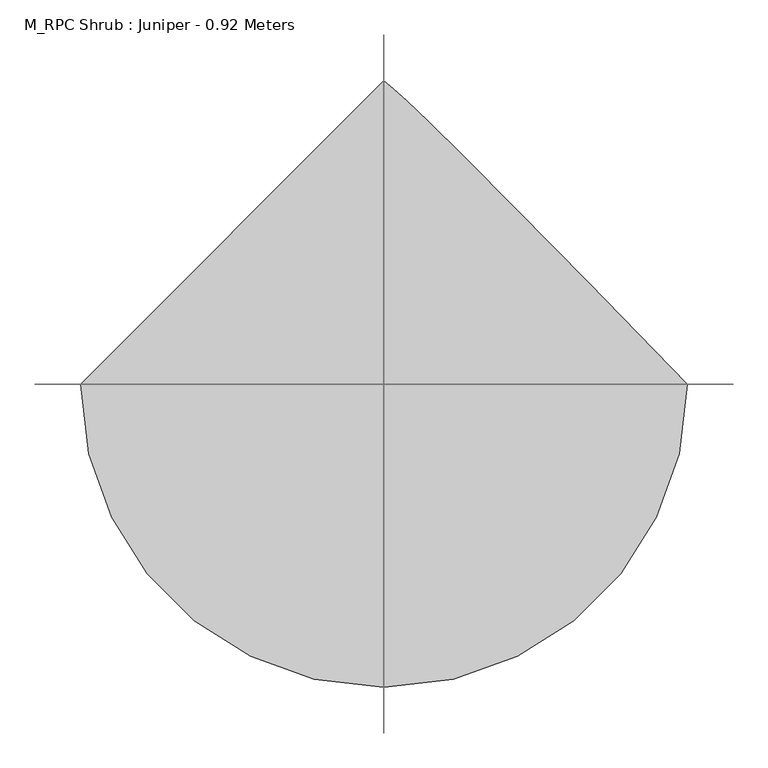
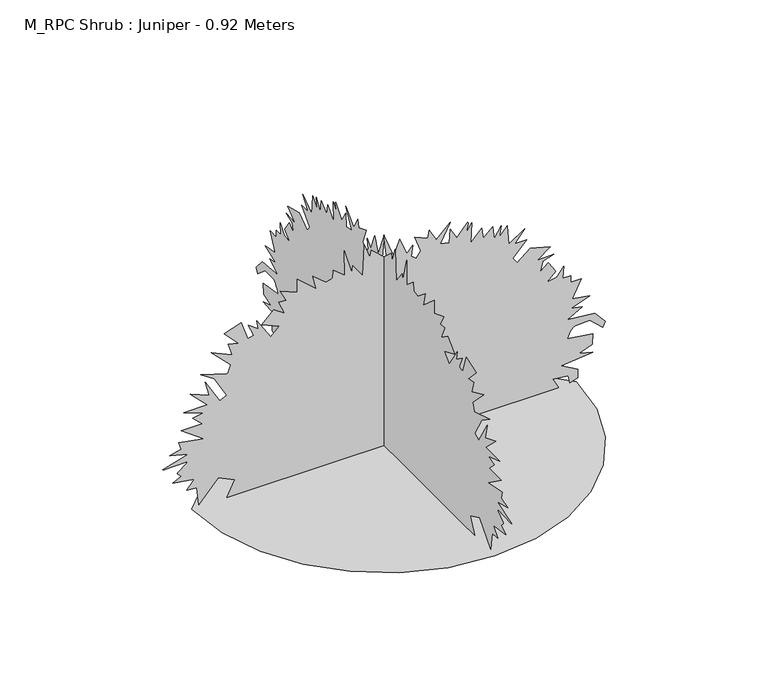
"""IFC4 building model written with IfcOpenShell, lengths in millimetres: geographic element geometry, M_RPC Shrub : Juniper - 0.92 Meters."""

from ifc_helpers import new_model, si_unit, origin, place, context, project, spatial, triangles, source, transform, mapped, element, save


def m_rpc_shrub_juniper_0_92_meters_8f64cf4e(model_context):
    return source(origin(), model_context, "Body", "Tessellation", [
        triangles([(-794.7784498, 0.0, 7.39e-05), (-773.7691944, -182.1108318, 7.39e-05), (-713.9282249, -349.3498243, 7.39e-05), (-620.0497982, -496.928171, 7.39e-05), (-496.928171, -620.0497982, 7.39e-05), (-349.3498243, -713.9282249, 7.39e-05), (-182.1108318, -773.7691944, 7.39e-05), (3.47e-05, -794.7784498, 7.39e-05), (182.1110862, -773.7691944, 7.39e-05), (349.3498243, -713.9282249, 7.39e-05), (496.928171, -620.0497982, 7.39e-05), (620.0497982, -496.928171, 7.39e-05), (713.9282249, -349.3498243, 7.39e-05), (773.7691944, -182.1108318, 7.39e-05), (794.7784498, 6.95e-05, 7.39e-05), (536.4933068, 264.9372079, 7.39e-05), (345.0130614, 460.0003741, 7.39e-05), (209.2048539, 596.8325744, 7.39e-05), (117.9336172, 687.0795731, 7.39e-05), (60.065061, 742.3894964, 7.39e-05), (24.4653762, 774.4080362, 7.39e-05), (-0.0001042, 794.7784498, 7.39e-05), (-3.6e-06, -649.9319859, 2.9e-06), (1e-06, -617.9951271, 67.2298217), (0.0, -685.063199, 99.2021479), (0.0, -764.9065086, 9.7766686), (0.0, -774.4898626, 86.4271646), (0.0, -816.0074593, 89.6208469), (0.0, -784.0706005, 127.946033), (0.0, -873.4947206, 140.7212706), (0.0, -838.3634348, 159.8838637), (0.0, -854.3330996, 175.8527654), (2e-07, -852.2145515, 179.4443521), (-1e-07, -815.0695078, 209.220696), (0.0, -812.8129595, 214.1779515), (2e-07, -908.8278111, 211.8641574), (0.0, -915.0148607, 214.1779515), (0.0, -809.6210758, 246.115537), (0.0, -886.2699583, 265.2771036), (0.0, -838.3634348, 278.0523412), (0.0, -847.9442453, 309.9916889), (0.0, -745.7449602, 290.8275607), (0.0, -838.3634348, 357.8981761), (0.0, -752.131271, 357.8981761), (0.0, -790.4569839, 396.2238891), (0.0, -745.7449602, 405.8046633), (0.0, -828.7826969, 434.5470222), (0.0, -729.7752228, 434.5470222), (0.0, -800.0377218, 504.8120647), (0.0, -723.388912, 472.8726989), (0.0, -739.3585768, 536.7488872), (0.0, -678.6743448, 434.5470222), (0.0, -649.9319859, 447.3222599), (0.0, -701.0328638, 536.7488872), (0.0, -758.5201979, 575.0745638), (0.0, -646.7374861, 539.9433143), (0.0, -633.9623211, 575.0745638), (0.0, -713.8081015, 654.9178734), (0.0, -627.5759377, 616.5921604), (0.0, -643.5456024, 667.693111), (0.0, -602.0254987, 658.1123005), (0.0, -659.5127237, 718.793989), (0.0, -589.250261, 744.3444643), (0.0, -563.6997857, 664.4986113), (0.0, -538.1493104, 670.8875381), (0.0, -560.5053223, 721.9859453), (0.0, -518.987762, 693.2435863), (6e-07, -525.3740727, 728.7095901), (0.0, -467.8868114, 638.9482086), (0.0, -432.7555618, 674.0794218), (0.0, -506.2125243, 706.0187513), (0.0, -455.1115737, 753.9252748), (0.0, -410.39955, 721.9859453), (0.0, -435.9500253, 779.4757502), (0.0, -404.0106594, 776.2813231), (0.0, -429.5611347, 824.1877739), (0.0, -359.2986357, 795.4428715), (0.0, -359.2986357, 852.9326763), (0.0, -279.4553261, 782.6676338), (0.0, -295.4224656, 843.3493223), (0.0, -241.1293769, 798.6372986), (0.0, -212.3857462, 805.0262255), (0.0, -209.1915553, 840.1574387), (0.0, -161.2850681, 801.8317257), (0.0, -164.4792591, 910.4199377), (0.0, -132.5414374, 801.8317257), (0.0, -129.3475008, 830.5740847), (0.0, -87.8283782, 773.0868233), (0.0, -81.4410228, 907.2255106), (0.0, -59.0844931, 843.3493223), (0.0, -52.6971332, 872.0942247), (0.0, 11.1781115, 814.6069633), (0.0, -1.5967073, 920.0007483), (0.0, 39.9224087, 814.6069633), (0.0, 65.4723617, 878.4806082), (0.0, 94.2162513, 805.0262255), (0.0, 119.7664632, 833.7685844), (0.0, 113.3788444, 789.056488), (0.0, 132.5416918, 773.0868233), (0.0, 151.7042848, 798.6372986), (0.0, 126.154082, 865.707914), (0.0, 180.448179, 843.3493223), (0.0, 186.8352891, 875.2887245), (0.0, 215.5796828, 824.1877739), (0.0, 273.0664355, 881.6750353), (0.0, 231.5483484, 801.8317257), (0.0, 269.8745519, 792.2509878), (0.0, 273.0664355, 849.7382492), (0.0, 301.8113561, 801.8317257), (0.0, 344.4942704, 854.0673454), (0.0, 346.8402755, 853.8730986), (0.0, 347.5124002, 849.9043728), (0.0, 340.1370509, 811.4125362), (0.0, 362.4930628, 846.5438221), (0.0, 359.2986357, 760.3115856), (0.0, 404.0132029, 808.2181091), (0.0, 410.39955, 763.5060854), (0.0, 448.7252629, 798.6372986), (0.0, 455.1115737, 744.3444643), (0.0, 483.8565125, 792.2509878), (0.0, 477.4676219, 744.3444643), (0.0, 509.4069514, 782.6676338), (0.0, 515.7932985, 699.6298971), (0.0, 582.8639139, 744.3444643), (0.0, 541.3437738, 693.2435863), (0.0, 589.250261, 693.2435863), (0.0, 531.7629633, 632.5618252), (0.0, 550.9245481, 607.0113862), (0.0, 605.2199258, 651.7234463), (0.0, 688.2576262, 629.3673981), (0.0, 633.9623211, 587.8498014), (0.0, 701.0328638, 591.0416851), (0.0, 656.3208401, 575.0745638), (0.0, 646.7374861, 533.5544237), (0.0, 678.6768883, 562.2993261), (0.0, 710.6136744, 514.392839), (0.0, 672.2879614, 479.2615894), (0.0, 713.8081015, 485.6479365), (0.0, 742.5504604, 523.9736495), (0.0, 739.3585768, 472.8726989), (0.0, 771.2953629, 472.8726989), (0.0, 771.2953629, 444.1303399), (0.0, 816.0074593, 444.1303399), (0.0, 777.6817463, 370.6734138), (0.0, 851.1386724, 357.8981761), (0.0, 774.4898626, 329.1532737), (0.0, 819.2018864, 319.5724631), (0.0, 758.5201979, 284.4412318), (0.0, 870.302837, 274.8604394), (0.0, 915.0148607, 223.7592526), (0.0, 905.4340502, 201.402732), (0.0, 851.1386724, 249.3092192), (0.0, 790.1144903, 247.912593), (0.0, 782.0312628, 244.0018215), (0.0, 775.4865314, 237.9960108), (0.0, 770.1683968, 230.3142667), (0.0, 765.7728075, 221.375441), (0.0, 761.993169, 211.5986395), (0.0, 758.5201979, 201.402732), (0.0, 863.9139101, 185.4340665), (0.0, 860.7220264, 140.7212706), (0.0, 806.4266487, 121.5586776), (0.0, 863.9139101, 105.5897668), (0.0, 732.9697226, 92.8147835), (0.0, 800.0403379, 54.489343), (0.0, 800.0403379, 16.164208), (0.0, 768.1009357, 6.582912), (0.0, 761.714625, 38.5206865), (0.0, 697.8384367, 44.9080465), (0.0, 723.388912, 0.1953706), (-649.9319859, 0.0001197, 0.0), (-617.9951271, 0.0001111, 67.2298217), (-685.063199, 0.0001102, 99.2021479), (-764.9065086, 0.0001155, 9.7766686), (-774.4898626, 0.0001109, 86.4271646), (-816.0074593, 0.0001107, 89.6208469), (-784.0706005, 0.0001084, 127.946033), (-873.4947206, 0.0001077, 140.7212706), (-838.3634348, 0.0001065, 159.8838637), (-854.3330996, 0.0001056, 175.8527654), (-852.2145515, 0.0001052, 179.4443521), (-815.0695078, 0.0001037, 209.220696), (-812.8129595, 0.0001033, 214.1779515), (-908.8278111, 0.0001032, 211.8641574), (-915.0148607, 0.0001033, 214.1779515), (-809.6210758, 0.0001014, 246.115537), (-886.2699583, 0.0001003, 265.2771036), (-838.3634348, 9.95e-05, 278.0523412), (-847.9442453, 9.76e-05, 309.9916889), (-745.7449602, 9.87e-05, 290.8275607), (-838.3634348, 9.47e-05, 357.8981761), (-752.131271, 9.47e-05, 357.8981761), (-790.4569839, 9.25e-05, 396.2238891), (-745.7449602, 9.19e-05, 405.8046633), (-828.7826969, 9.02e-05, 434.5470222), (-729.7752228, 9.02e-05, 434.5470222), (-800.0377218, 8.6e-05, 504.8095213), (-723.388912, 8.79e-05, 472.8726989), (-739.3585768, 8.41e-05, 536.7488872), (-678.6768883, 9.02e-05, 434.5470222), (-649.9319859, 8.94e-05, 447.3222599), (-701.0328638, 8.41e-05, 536.7488872), (-758.5201979, 8.18e-05, 575.0745638), (-646.7374861, 8.39e-05, 539.9433143), (-633.9623211, 8.18e-05, 575.0745638), (-713.8081015, 7.7e-05, 654.9178734), (-627.5759377, 7.93e-05, 616.5921604), (-643.5456024, 7.63e-05, 667.693111), (-602.0254987, 7.68e-05, 658.1123005), (-659.5127237, 7.32e-05, 718.793989), (-589.250261, 7.17e-05, 744.3444643), (-563.6997857, 7.65e-05, 664.4986113), (-538.1493104, 7.61e-05, 670.8875381), (-560.5053223, 7.3e-05, 721.9859453), (-518.987762, 7.48e-05, 693.2435863), (-525.3740727, 7.2e-05, 728.7095901), (-467.8868114, 7.8e-05, 638.9482086), (-432.7555618, 7.59e-05, 674.0794218), (-506.2125243, 7.4e-05, 706.0187513), (-455.1115737, 7.11e-05, 753.9252748), (-410.39955, 7.3e-05, 721.9859453), (-435.9500253, 6.96e-05, 779.4757502), (-404.0132029, 6.98e-05, 776.2813231), (-429.5611347, 6.69e-05, 824.1877739), (-359.2986357, 6.87e-05, 795.4428715), (-359.2986357, 6.52e-05, 852.9326763), (-279.4553261, 6.94e-05, 782.6676338), (-295.4224656, 6.58e-05, 843.3493223), (-241.1293769, 6.85e-05, 798.6372986), (-212.3857462, 6.81e-05, 805.0262255), (-209.1918097, 6.6e-05, 840.1574387), (-161.2850681, 6.83e-05, 801.8317257), (-164.4792591, 6.18e-05, 910.4199377), (-132.5416918, 6.83e-05, 801.8317257), (-129.3475008, 6.66e-05, 830.5740847), (-87.8286325, 7e-05, 773.0868233), (-81.4410228, 6.2e-05, 907.2255106), (-59.0847475, 6.58e-05, 843.3493223), (-52.6973875, 6.41e-05, 872.0942247), (11.1780093, 6.75e-05, 814.6069633), (-1.5967993, 6.12e-05, 920.0007483), (39.9221544, 6.75e-05, 814.6069633), (65.4723617, 6.37e-05, 878.4806082), (94.2162513, 6.81e-05, 805.0262255), (119.7664632, 6.64e-05, 833.7685844), (113.3788444, 6.9e-05, 789.056488), (132.5414374, 7e-05, 773.0868233), (151.7040305, 6.85e-05, 798.6372986), (126.154082, 6.45e-05, 865.7053705), (180.4479246, 6.58e-05, 843.3493223), (186.8352891, 6.39e-05, 875.2887245), (215.5794285, 6.69e-05, 824.1877739), (273.0664355, 6.35e-05, 881.6750353), (231.5483484, 6.83e-05, 801.8317257), (269.8745519, 6.89e-05, 792.2509878), (273.0664355, 6.54e-05, 849.7382492), (301.8113561, 6.83e-05, 801.8317257), (344.4942704, 6.52e-05, 854.0673454), (346.8402755, 6.52e-05, 853.8730986), (347.5098204, 6.54e-05, 849.9043728), (340.1370509, 6.77e-05, 811.4125362), (362.4930628, 6.56e-05, 846.5438221), (359.2986357, 7.08e-05, 760.3115856), (404.0106594, 6.79e-05, 808.2181091), (410.39955, 7.06e-05, 763.5060854), (448.7252629, 6.85e-05, 798.6372986), (455.1115737, 7.17e-05, 744.3444643), (483.8565125, 6.89e-05, 792.2509878), (477.4676219, 7.17e-05, 744.3444643), (509.4069514, 6.94e-05, 782.6676338), (515.7932985, 7.44e-05, 699.6298971), (582.8639139, 7.17e-05, 744.3444643), (541.3437738, 7.48e-05, 693.2435863), (589.250261, 7.48e-05, 693.2435863), (531.7629633, 7.84e-05, 632.5618252), (550.9245481, 7.99e-05, 607.0113862), (605.2199258, 7.72e-05, 651.7234463), (688.2576262, 7.86e-05, 629.3673981), (633.9623211, 8.1e-05, 587.8498014), (701.0328638, 8.08e-05, 591.0416851), (656.3208401, 8.18e-05, 575.0745638), (646.7374861, 8.43e-05, 533.5544237), (678.6768883, 8.26e-05, 562.2993261), (710.6136744, 8.54e-05, 514.392839), (672.2879614, 8.75e-05, 479.2615894), (713.8081015, 8.71e-05, 485.6479365), (742.5504604, 8.48e-05, 523.9736495), (739.3585768, 8.79e-05, 472.8726989), (771.2953629, 8.79e-05, 472.8726989), (771.2953629, 8.96e-05, 444.1303399), (816.0074593, 8.96e-05, 444.1303399), (777.6817463, 9.4e-05, 370.6734138), (851.1386724, 9.47e-05, 357.8981761), (774.4898626, 9.65e-05, 329.1532737), (819.2018864, 9.7e-05, 319.5724631), (758.5201979, 9.91e-05, 284.4412318), (870.302837, 9.97e-05, 274.8604394), (915.0148607, 0.0001027, 223.7592526), (905.4340502, 0.0001041, 201.402732), (851.1386724, 0.0001012, 249.3092192), (790.1144903, 0.0001013, 247.912593), (782.0312628, 0.0001015, 244.0018215), (775.4865314, 0.0001019, 237.9960108), (770.1683968, 0.0001023, 230.3142667), (765.7728075, 0.0001029, 221.375441), (761.993169, 0.0001035, 211.5986395), (758.5201979, 0.0001041, 201.402732), (863.9139101, 0.000105, 185.4338121), (860.7220264, 0.0001077, 140.7212706), (806.4266487, 0.0001088, 121.5586776), (863.9139101, 0.0001098, 105.5897668), (732.9697226, 0.0001105, 92.8145291), (800.0403379, 0.0001128, 54.489343), (800.0403379, 0.0001151, 16.164208), (768.1009357, 0.0001157, 6.582912), (761.714625, 0.0001138, 38.5206865), (697.8384367, 0.0001134, 44.9080465), (723.388912, 0.0001161, 0.1953678)], [[21, 22, 1], [20, 21, 1], [19, 20, 1], [18, 19, 1], [17, 18, 1], [17, 1, 2], [17, 2, 3], [17, 3, 4], [16, 17, 4], [16, 4, 5], [16, 5, 6], [16, 6, 7], [16, 7, 8], [16, 8, 9], [16, 9, 10], [16, 10, 11], [16, 11, 12], [15, 16, 12], [14, 15, 12], [13, 14, 12], [92, 93, 94], [84, 85, 86], [54, 55, 56], [50, 51, 52], [131, 132, 133], [123, 124, 125], [104, 105, 106], [46, 47, 48], [57, 58, 59], [88, 89, 90], [48, 49, 50], [67, 68, 69], [119, 120, 121], [162, 163, 164], [38, 39, 40], [113, 114, 115], [144, 145, 146], [65, 66, 67], [138, 139, 140], [96, 97, 98], [107, 108, 109], [79, 80, 81], [42, 43, 44], [29, 30, 31], [36, 37, 38], [75, 76, 77], [102, 103, 104], [146, 147, 148], [86, 87, 88], [94, 95, 96], [121, 122, 123], [125, 126, 127], [100, 101, 102], [77, 78, 79], [25, 26, 27], [115, 116, 117], [129, 130, 131], [117, 118, 119], [27, 28, 29], [82, 83, 84], [44, 45, 46], [48, 50, 52], [59, 60, 61], [169, 170, 23], [73, 74, 75], [90, 91, 92], [142, 143, 144], [40, 41, 42], [38, 40, 42], [169, 23, 24], [53, 54, 56], [61, 62, 63], [61, 63, 64], [70, 71, 72], [70, 72, 73], [150, 151, 152], [149, 150, 152], [148, 149, 152], [148, 152, 153], [128, 129, 131], [148, 153, 154], [35, 36, 38], [134, 135, 136], [134, 136, 137], [65, 67, 69], [166, 167, 168], [165, 166, 168], [164, 165, 168], [164, 168, 169], [88, 90, 92], [140, 141, 142], [100, 102, 104], [159, 160, 161], [159, 161, 162], [25, 27, 29], [123, 125, 127], [148, 154, 155], [100, 104, 106], [110, 111, 112], [109, 110, 112], [109, 112, 113], [109, 113, 115], [31, 32, 33], [131, 133, 134], [159, 162, 164], [128, 131, 134], [46, 48, 52], [73, 75, 77], [73, 77, 79], [29, 31, 33], [29, 33, 34], [44, 46, 52], [148, 155, 156], [164, 169, 24], [159, 164, 24], [158, 159, 24], [157, 158, 24], [156, 157, 24], [148, 156, 24], [146, 148, 24], [144, 146, 24], [142, 144, 24], [140, 142, 24], [138, 140, 24], [137, 138, 24], [134, 137, 24], [128, 134, 24], [127, 128, 24], [123, 127, 24], [121, 123, 24], [119, 121, 24], [117, 119, 24], [115, 117, 24], [109, 115, 24], [107, 109, 24], [106, 107, 24], [106, 24, 25], [106, 25, 29], [106, 29, 34], [106, 34, 35], [106, 35, 38], [106, 38, 42], [106, 42, 44], [106, 44, 52], [106, 52, 53], [106, 53, 56], [99, 100, 106], [99, 106, 56], [99, 56, 57], [98, 99, 57], [96, 98, 57], [94, 96, 57], [59, 61, 64], [57, 59, 64], [70, 73, 79], [64, 65, 69], [57, 64, 69], [94, 57, 69], [84, 86, 88], [88, 92, 94], [88, 94, 69], [88, 69, 70], [88, 70, 79], [84, 88, 79], [82, 84, 79], [82, 79, 81], [240, 241, 242], [232, 233, 234], [202, 203, 204], [198, 199, 200], [279, 280, 281], [271, 272, 273], [252, 253, 254], [194, 195, 196], [205, 206, 207], [236, 237, 238], [196, 197, 198], [215, 216, 217], [267, 268, 269], [310, 311, 312], [186, 187, 188], [261, 262, 263], [292, 293, 294], [213, 214, 215], [286, 287, 288], [244, 245, 246], [255, 256, 257], [227, 228, 229], [190, 191, 192], [177, 178, 179], [184, 185, 186], [223, 224, 225], [250, 251, 252], [294, 295, 296], [234, 235, 236], [242, 243, 244], [269, 270, 271], [273, 274, 275], [248, 249, 250], [225, 226, 227], [173, 174, 175], [263, 264, 265], [277, 278, 279], [265, 266, 267], [175, 176, 177], [230, 231, 232], [192, 193, 194], [196, 198, 200], [207, 208, 209], [317, 318, 171], [221, 222, 223], [238, 239, 240], [290, 291, 292], [188, 189, 190], [186, 188, 190], [317, 171, 172], [201, 202, 204], [209, 210, 211], [209, 211, 212], [218, 219, 220], [218, 220, 221], [298, 299, 300], [297, 298, 300], [296, 297, 300], [296, 300, 301], [276, 277, 279], [296, 301, 302], [183, 184, 186], [282, 283, 284], [282, 284, 285], [213, 215, 217], [314, 315, 316], [313, 314, 316], [312, 313, 316], [312, 316, 317], [236, 238, 240], [288, 289, 290], [248, 250, 252], [307, 308, 309], [307, 309, 310], [173, 175, 177], [271, 273, 275], [296, 302, 303], [248, 252, 254], [258, 259, 260], [257, 258, 260], [257, 260, 261], [257, 261, 263], [179, 180, 181], [279, 281, 282], [307, 310, 312], [276, 279, 282], [194, 196, 200], [221, 223, 225], [221, 225, 227], [177, 179, 181], [177, 181, 182], [192, 194, 200], [296, 303, 304], [312, 317, 172], [307, 312, 172], [306, 307, 172], [305, 306, 172], [304, 305, 172], [296, 304, 172], [294, 296, 172], [292, 294, 172], [290, 292, 172], [288, 290, 172], [286, 288, 172], [285, 286, 172], [282, 285, 172], [276, 282, 172], [275, 276, 172], [271, 275, 172], [269, 271, 172], [267, 269, 172], [265, 267, 172], [263, 265, 172], [257, 263, 172], [255, 257, 172], [254, 255, 172], [254, 172, 173], [254, 173, 177], [254, 177, 182], [254, 182, 183], [254, 183, 186], [254, 186, 190], [254, 190, 192], [254, 192, 200], [254, 200, 201], [254, 201, 204], [247, 248, 254], [247, 254, 204], [247, 204, 205], [246, 247, 205], [244, 246, 205], [242, 244, 205], [207, 209, 212], [205, 207, 212], [218, 221, 227], [212, 213, 217], [205, 212, 217], [242, 205, 217], [232, 234, 236], [236, 240, 242], [236, 242, 217], [236, 217, 218], [236, 218, 227], [232, 236, 227], [230, 232, 227], [230, 227, 229]], closed=False),
    ])


if __name__ == "__main__":
    model = new_model("IFC4")
    model_context = context("Model", 3, world=origin())
    ifc_project = project(units=[si_unit("LENGTHUNIT", "METRE", prefix="MILLI")], contexts=[model_context])
    site = spatial("IfcSite", under=ifc_project)
    building = spatial("IfcBuilding", under=site)
    placement = place(None, origin())
    m_rpc_shrub_juniper_0_92_meters_shape = m_rpc_shrub_juniper_0_92_meters_8f64cf4e(model_context)
    element("IfcGeographicElement", 1, ObjectType="M_RPC Shrub : Juniper - 0.92 Meters", at=placement, inside=building, context=model_context, shape_type="MappedRepresentation", body=[
        mapped(m_rpc_shrub_juniper_0_92_meters_shape, transform((0.0, 0.0, 0.0), x_axis=(1.0, 0.0, 0.0), y_axis=(0.0, 1.0, 0.0), z_axis=(0.0, 0.0, 1.0))),
    ])
    save(model, "model.ifc")

# Revit data of these elements
# Type "M_RPC Shrub : Juniper - 0.92 Meters"
#   Type Comments = "Juniper"
#   built-in parameter 1005198 = "{2, 15},{39, RPC-16-FU4H-UTPX-8HVP-A000-ST1L-LVER-AU},{1, 0},{1, 0},{2, 35},{1, 8},{5, Color},{1, 0},{1, 0},{3, 0.8},{3, 0.8},{3, 0.8},{1, 8},{7, BBoxMin},{1, 0},{1, 0},{1, 0},{1, 0},{1, 0},{1, 8},{7, BBoxMax},{1, 0},{1, 0},{1, 0},{1, 0},{1, 0},{2, 11},{9, RPCTypeId},{1, 0},{1, 0},{39, RPC-16-FU4H-UTPX-8HVP-A000-ST1L-LVER-AU},{1, 6},{14, RPCPlantHeight},{1, 0},{1, 0},{7, 3.01837},{2, 11},{7, keyword},{1, 0},{1, 0},{21, :Geometry:RPC:Juniper},{2, 11},{8, category},{1, 0},{1, 0},{17, :Shrubs & Grasses},{2, 11},{12, LocalizedUID},{1, 0},{1, 0},{7, Juniper},{2, 14},{6, Height},{1, 0},{1, 0},{7, 3.01837},{1, 2},{16, Cast Reflections},{1, 0},{1, 0},{1, 0},{1, 2},{12, Cast Shadows},{1, 0},{1, 0},{1, 1},{1, 2},{9, Lock View},{1, 0},{1, 0},{1, 0},{1, 4},{5, ViewC},{1, 0},{1, 0},{1, 0},{2, 11},{20, AdvancedUIDefinition},{1, 0},{1, 0},{0, },{2, 11},{10, AssetLibID},{1, 0},{1, 0},{36, 4D3F6E72-3F99-4203-98E9-AF80B3C7A7A4},{2, 11},{10, BaseSchema},{1, 0},{1, 0},{9, RPCSchema},{2, 11},{12, ExchangeGUID},{1, 0},{1, 0},{0, },{1, 2},{6, Hidden},{1, 0},{1, 0},{1, 0},{1, 4},{11, RPCCategory},{1, 0},{1, 0},{1, 0},{2, 11},{8, RPCImage},{1, 0},{1, 0},{0, },{1, 4},{13, SchemaVersion},{1, 0},{1, 0},{1, 4},{2, 11},{12, UIDefinition},{1, 0},{1, 0},{0, },{2, 11},{6, UIName},{1, 0},{1, 0},{39, RPC-16-FU4H-UTPX-8HVP-A000-ST1L-LVER-AU},{2, 11},{11, VersionGUID},{1, 0},{1, 0},{9, RPCSchema},{2, 11},{9, assettype},{1, 0},{1, 0},{11, RPCGeometry},{2, 11},{11, description},{1, 0},{1, 0},{0, },{2, 11},{9, localname},{1, 0},{1, 0},{3, RPC},{2, 11},{9, localtype},{1, 0},{1, 0},{3, RPC},{1, 4},{8, revision},{1, 0},{1, 0},{1, 1},{2, 11},{9, thumbnail},{1, 0},{1, 0},{0, },{1, 4},{7, version},{1, 0},{1, 0},{1, 1},{1, 2},{20, RPC_Cast Reflections},{1, 0},{1, 0},{1, 1},{1, 2},{16, RPC_Cast Shadows},{1, 0},{1, 0},{1, 1},{1, 2},{13, RPC_Lock View},{1, 0},{1, 0},{1, 0},{1, 4},{9, RPC_ViewC},{1, 0},{1, 0},{1, 0},{21, assetlibrary_base.fbx},{1, 5},"
#   built-in parameter 1005195 = "RPC-16-FU4H-UTPX-8HVP-A000-ST1L-LVER-AU"
#   Height = 920 mm
#   Description = (empty or 0)
#   Default Elevation = 0
